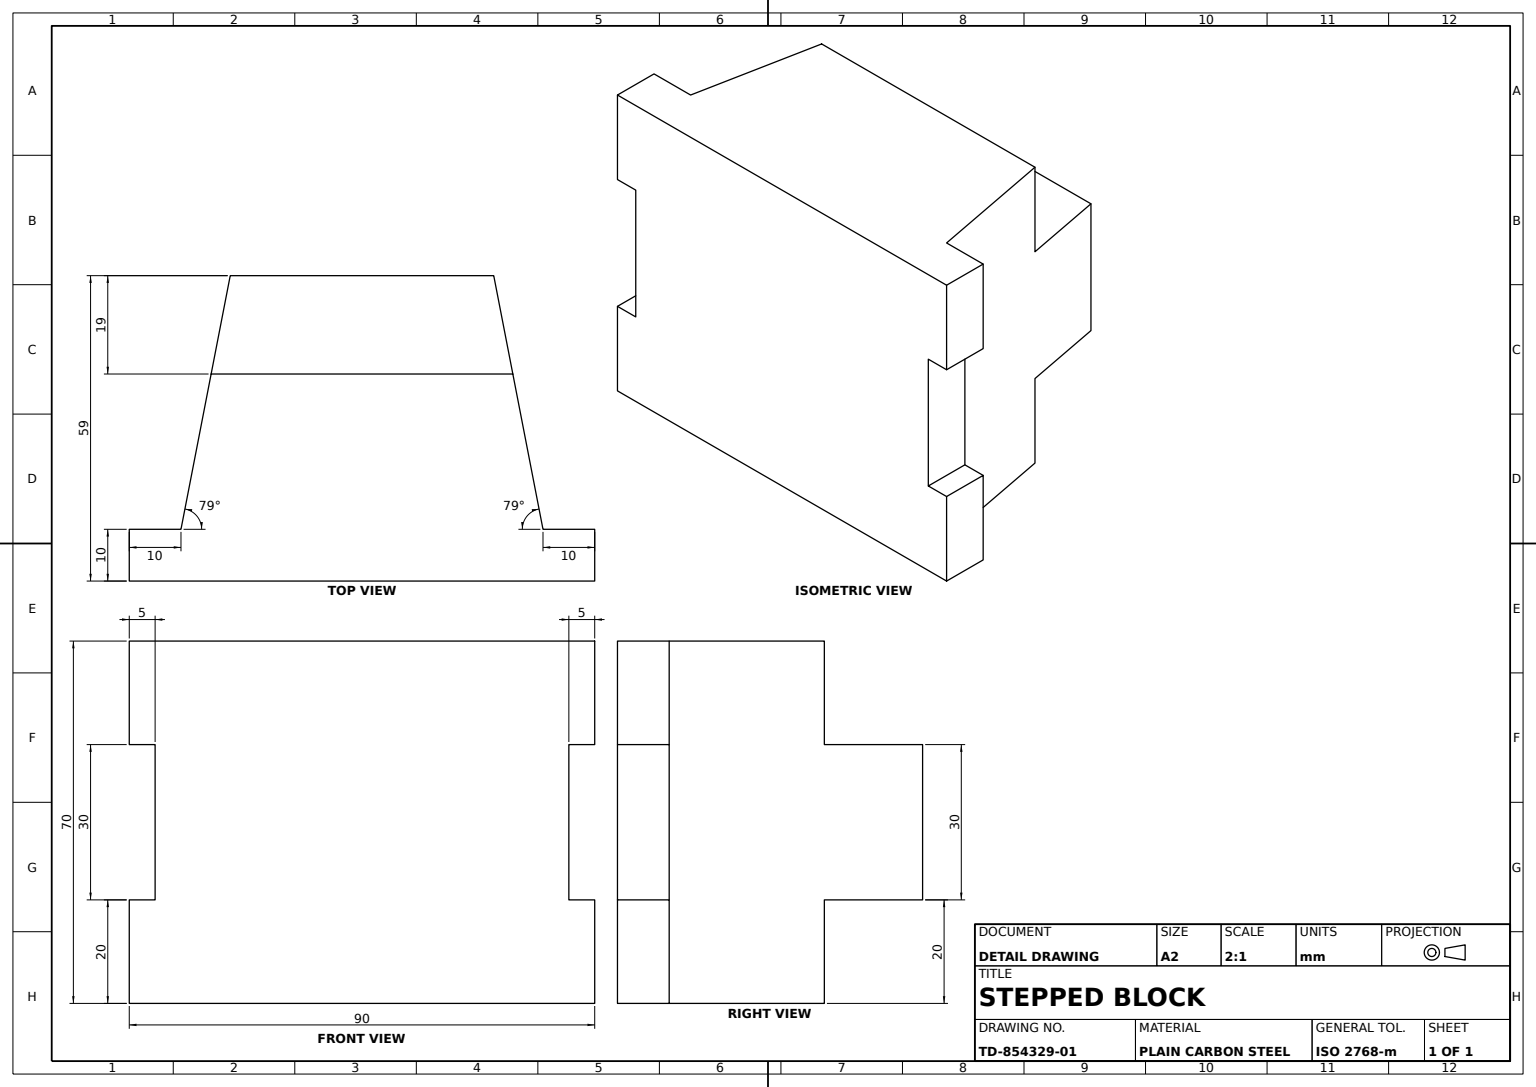
SolidWorks part; units mm, degrees
material "Plain Carbon Steel"
ref_plane "Front Plane" through (0, 0, 0) normal (0, 0, 1) x (1, 0, 0)
ref_plane "Top Plane" through (0, 0, 0) normal (0, 1, 0) x (1, 0, 0)
ref_plane "Right Plane" through (0, 0, 0) normal (1, 0, 0) x (0, 0, -1)
sketch "Base Plate Profile" plane through (0, 0, 0) normal (0, 0, 1) x (1, 0, 0)
  line L0 (-45, -15) -> (-45, -35)
  line L1 (-45, 35) -> (45, 35)
  line L2 (-45, 35) -> (-45, 15)
  line L3 (-45, -35) -> (45, -35)
  line L4 (45, 35) -> (45, 15)
  line L5 (-45, 35) -> (45, -35) construction
  line L6 (-45, -35) -> (45, 35) construction
  line L7 (-45, 15) -> (-40, 15)
  line L9 (-45, -15) -> (-40, -15)
  line L10 (-40, 15) -> (-40, -15)
  line L11 (45, 15) -> (40, 15)
  line L13 (45, -15) -> (40, -15)
  line L14 (40, 15) -> (40, -15)
  line L15 (45, -15) -> (45, -35)
  point P0 (0, 0)
  dimension "D1" = 90
  dimension "D2" = 70
  dimension "D3" = 30
  dimension "D4" = 5
  dimension "D5" = 30
  dimension "D6" = 5
  dimension "D7" = 20
  dimension "D8" = 20
extrude "Base Plate" add sketch "Base Plate Profile" along normal blind 10
sketch "Tapered Boss Profile" plane through (0, 35, 0) normal (0, 1, 0) x (1, 0, 0)
  line L0 (-25.4754, 49) -> (-35, 0)
  line L1 (35, 0) -> (25.4754, 49)
  line L2 (-35, 0) -> (35, 0)
  line L3 (45, 0) -> (-45, 0) construction
  line L4 (-25.4754, 49) -> (25.4754, 49)
  line L6 (-45, -10) -> (-45, 0) construction
  line L7 (45, -10) -> (45, 0) construction
  dimension "D2" = 79
  dimension "D3" = 79
  dimension "D4" = 70
  dimension "D5" = 10
  dimension "D6" = 10
  dimension "D7" = 49
extrude "Tapered Boss" add sketch "Tapered Boss Profile" against normal up to surface (70 mm away) up to face at (0, -35, 5)
sketch "Top Slot Profile" plane through (0, 0, -49) normal (0, 0, -1) x (-1, 0, 0)
  line L0 (-25.4754, 35) -> (25.4754, 35) construction
  line L1 (-38.9138, 35) -> (53.5134, 35)
  line L2 (-38.9138, 35) -> (-38.9138, 15)
  line L3 (-38.9138, 15) -> (53.5134, 15)
  line L4 (53.5134, 35) -> (53.5134, 15)
  line L5 (-38.9138, -35) -> (51.0735, -35)
  line L6 (-38.9138, -35) -> (-38.9138, -15)
  line L7 (-38.9138, -15) -> (51.0735, -15)
  line L8 (51.0735, -35) -> (51.0735, -15)
  line L9 (25.4754, -35) -> (-25.4754, -35) construction
  line L10 (25.4754, -35) -> (25.4754, 35) construction
  dimension "D1" = 20
  dimension "D2" = 20
  dimension "D3" = 0
  dimension "D4" = 0
  dimension "D5" = 25.5982
  dimension "D6" = 28.038
  dimension "D7" = 64.3892
extrude "Top Slot Cut 19mm" cut sketch "Top Slot Profile" against normal blind 19
